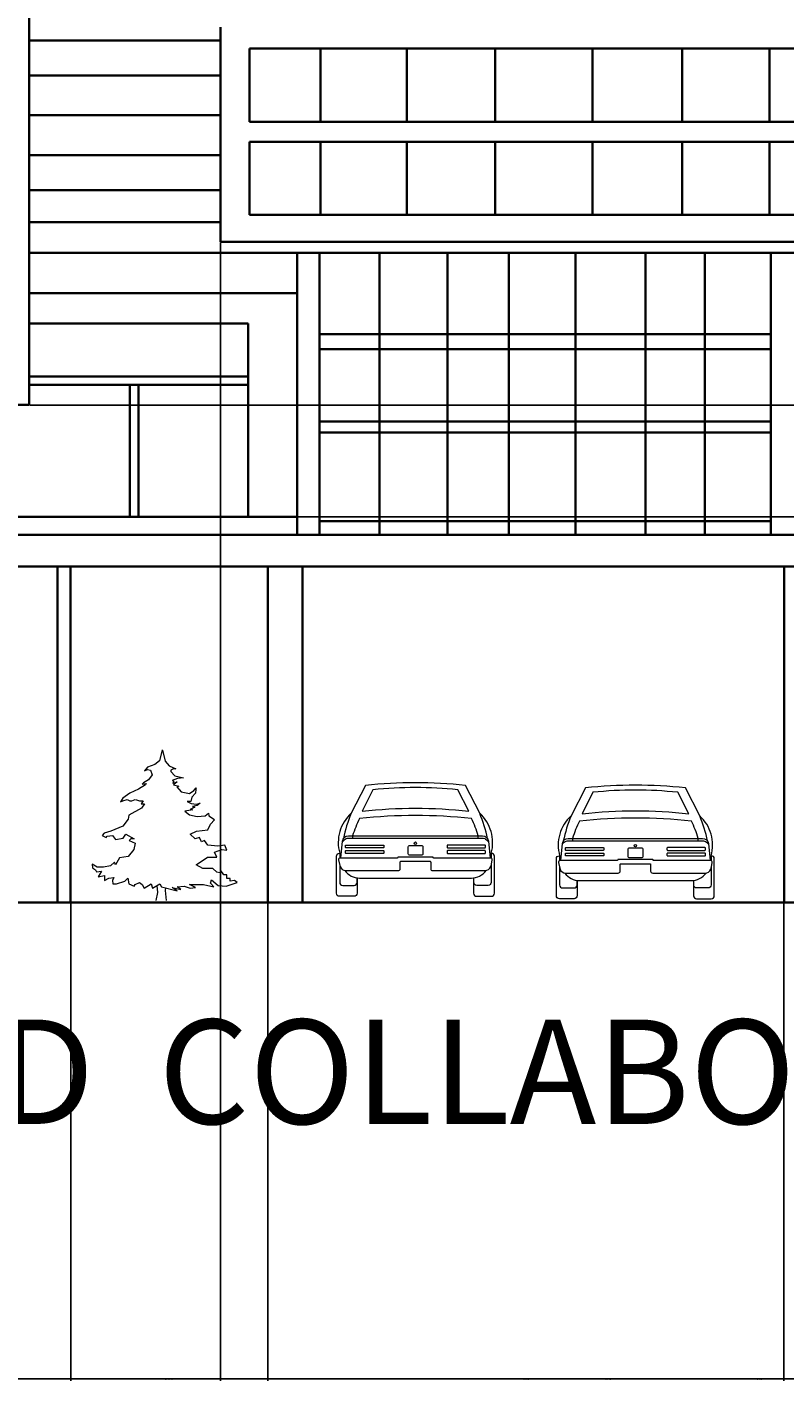
# Model space of a CAD drawing. Units: inches. Extents: x -160 to 434, y -145 to 103.
# Tile 4 of 7: x 107 to 176, y -145 to -22. Entities that reach past the tile are written whole.
import ezdxf

# ---------------------------------------------------------------- set-up
doc = ezdxf.new("R2010")
doc.units = ezdxf.units.IN
doc.header["$MEASUREMENT"] = 0
for name, color, linetype, lineweight in [('A-ANNO-DIMS', 2, 'Continuous', 18), ('A-ANNO-TEXT', 3, 'Continuous', 18), ('A-ELEV', 7, 'Continuous', 35), ('A-ENTO-VEHC', 8, 'Continuous', 13), ('L-PLNT', 3, 'Continuous', 13)]:
    doc.layers.add(name, color=color, linetype=linetype, lineweight=lineweight)
doc.styles.get("Standard").update_dxf_attribs({"font": 'arial.ttf'})
doc.dimstyles.get("Standard").update_dxf_attribs({"dimtxt": 0.18, "dimasz": 0.18, "dimexe": 0.18, "dimexo": 0.0625, "dimgap": 0.09, "dimtad": 0, "dimtih": 1, "dimtoh": 1, "dimdec": 4, "dimzin": 0, "dimdsep": 46, "dimtxsty": 'Standard', "dimcen": 0.09, "dimadec": 0, "dimazin": 0, "dimtfac": 1, "dimtdec": 4, "dimtofl": 0, "dimtmove": 0, "dimatfit": 3, "dimfxl": 1, "dimtolj": 1, "dimtzin": 0, "dimarcsym": 0})

# ---------------------------------------------------------------- blocks, each defined once
blk = doc.blocks.new('*U6')
for p, q in [((-24.66, 54.68), (-31.66, 40.93)), ((31.66, 40.93), (24.66, 54.68)), ((-30.95, 37.96), (-30.95, 37.96)), ((-37.32, 21.22), (-36.82, 18.83)), ((36.82, 18.83), (37.31, 21.2)), ((-27.55, 9), (27.55, 9))]:
    blk.add_line(p, q)
for points in [[(-20.92, 52.5), (-26.31, 41.89), (-26.31, 41.89, -0.059427), (26.31, 41.89), (20.92, 52.5, 0.05217)], [(-34.12, 25.29), (-15.92, 25.29, -0.414214), (-15.55, 24.92), (-15.55, 24.24, -0.414214), (-15.92, 23.87), (-34.12, 23.87, -0.414214), (-34.49, 24.24), (-34.49, 24.92, -0.414214)], [(-34.12, 22.54), (-15.92, 22.54, -0.414214), (-15.55, 22.17), (-15.55, 21.49, -0.414214), (-15.92, 21.12), (-34.12, 21.12, -0.414214), (-34.49, 21.49), (-34.49, 22.17, -0.414214)], [(-2.82, 25.12), (2.9, 25.12, -0.414214), (3.64, 24.38), (3.64, 20.97, -0.414214), (2.9, 20.23), (-2.82, 20.23, -0.414214), (-3.56, 20.97), (-3.56, 24.38, -0.414214)], [(34.12, 25.29), (15.92, 25.29, 0.414214), (15.55, 24.92), (15.55, 24.24, 0.414214), (15.92, 23.87), (34.12, 23.87, 0.414214), (34.49, 24.24), (34.49, 24.92, 0.414214)], [(34.12, 22.54), (15.92, 22.54, 0.414214), (15.55, 22.17), (15.55, 21.49, 0.414214), (15.92, 21.12), (34.12, 21.12, 0.414214), (34.49, 21.49), (34.49, 22.17, 0.414214)], [(-7.5, 16.83, -0.414214), (-7, 17.33), (7, 17.33, -0.414214), (7.5, 16.83), (7.5, 13.67, 0.414214), (8.5, 12.67), (34.29, 12.67, 0.322734), (37.1, 14.69, 0.029256), (37.41, 15.83), (37.84, 17.94, 0.475639), (37.12, 18.83), (9, 18.83, -0.414214), (8.75, 19.08, 0.414214), (8.5, 19.33), (-8.5, 19.33, 0.414214), (-8.75, 19.08, -0.414214), (-9, 18.83), (-37.12, 18.83, 0.475639), (-37.84, 17.94), (-37.41, 15.83, 0.029158), (-37.1, 14.7, 0.322842), (-34.29, 12.67), (-8.5, 12.67, 0.414214), (-7.5, 13.67)]]:
    blk.add_lwpolyline(points, format="xyb", close=True)
for points in [[(30.95, 28.64), (30.95, 29.82, 0.037308), (27.62, 38.34, 0.052989), (-27.62, 38.34, 0.037308), (-30.95, 29.82), (-30.95, 28.64)], [(-36.82, 18.83), (-35.99, 27.2, -0.380946), (-33.05, 29.82), (33.04, 29.82, -0.380474), (35.98, 27.2), (36.82, 18.83)], [(-36.02, 26.89), (-35.02, 27.89, -0.184023), (-33.05, 28.64), (33.05, 28.64, -0.184023), (35.02, 27.89), (36.02, 26.89)], [(-28.73, 9.08), (-28.73, 1.48, -0.414214), (-30.21, 0), (-37.44, 0, -0.414214), (-38.92, 1.48), (-38.92, 19.74, -0.414214), (-37.44, 21.22), (-37.32, 21.22)], [(28.67, 9.07), (28.67, 1.48, 0.414214), (30.15, 0), (37.38, 0, 0.414214), (38.86, 1.48), (38.86, 19.74, 0.414214), (37.38, 21.22), (37.32, 21.22)], [(-37.32, 15.44), (-37.32, 6.85, 0.414214), (-35.84, 5.37), (-30.21, 5.37, 0.414214), (-28.73, 6.85), (-28.73, 9.08)], [(37.32, 15.44), (37.32, 6.85, -0.414214), (35.84, 5.37), (30.21, 5.37, -0.414214), (28.73, 6.85), (28.73, 9.08)]]:
    blk.add_lwpolyline(points, format="xyb")
for points in [[(-37.32, 21.22), (-37.32, 18.8)], [(37.32, 21.22), (37.32, 18.8)]]:
    blk.add_lwpolyline(points)
blk.add_circle((0, 26.18), 0.596)
for centre, radius, start, end in [((0, -181.13), 237.1, 84.03003, 95.96997), ((-18.4, 26.45), 19.63, 132.48354, 195.46582), ((30.86, 14.66), 67.81, 157.21243, 168.23657), ((18.26, 26.38), 19.77, 344.85949, 47.35975), ((-31.75, 14.41), 68.72, 11.82698, 22.66251), ((-27.55, 17.88), 8.88, 215.57759, 270.00275), ((27.55, 17.88), 8.88, 270.00275, 324.39991)]:
    blk.add_arc(centre, radius, start, end)
blk = doc.blocks.new('*U7')
for p, q in [((-8.263, 7.598), (-8.747, 14.105)), ((-9.75, 0), (-8.263, 7.598)), ((-0.771, 9.56), (-0.69, 11.833)), ((0, 0), (-0.771, 9.56))]:
    blk.add_line(p, q)
for points in [[(-3.9, 142.35), (-6.596, 132.037), (-10.801, 128.443), (-17.81, 126.047), (-20.614, 122.452), (-17.81, 123.65), (-15.007, 123.051), (-13.605, 118.858), (-16.876, 114.065), (-21.549, 111.07), (-22.951, 109.872), (-19.212, 110.471), (-19.68, 109.273), (-26.222, 105.079), (-34.633, 101.485), (-41.175, 96.693), (-43.511, 93.098), (-41.175, 94.296), (-36.969, 95.494), (-34.633, 94.296), (-32.764, 94.296), (-29.493, 95.494)], [(-3.759, 141.97), (-1.074, 131.643), (2.437, 127.141), (8.84, 124.493), (6.568, 124.493), (4.09, 123.169), (4.296, 121.846), (7.807, 117.874), (16.069, 116.02), (10.492, 115.226), (5.535, 113.372), (6.981, 112.843), (5.948, 110.989), (10.286, 112.048), (6.775, 109.401), (11.732, 108.077), (9.873, 107.282), (13.797, 102.516), (21.852, 101.192), (25.983, 103.84), (28.048, 106.488), (27.842, 105.164), (27.429, 101.457), (24.124, 97.75), (23.091, 93.513), (19.58, 93.513), (23.505, 91.66), (28.255, 90.866), (31.973, 91.925), (29.081, 89.806), (24.537, 88.747), (26.809, 88.218), (22.472, 86.099), (24.95, 85.57), (17.308, 84.246), (21.852, 80.804), (29.081, 79.215), (36.723, 80.009), (39.821, 82.392), (40.028, 80.009), (45.398, 76.567)], [(-29.25, 95.55), (-25.287, 94.296), (-22.016, 94.296), (-23.885, 91.301), (-20.614, 91.301), (-23.418, 87.108), (-35.567, 80.518), (-36.035, 76.924), (-41.175, 70.334), (-52.389, 65.542), (-58.931, 63.744), (-60.8, 61.348), (-57.062, 59.551), (-56.128, 60.749), (-50.987, 61.348), (-48.184, 57.754), (-40.707, 58.952), (-38.371, 62.546), (-30.427, 58.353), (-33.698, 58.353), (-35.1, 56.556), (-29.493, 54.159), (-30.894, 48.169), (-36.035, 41.579), (-44.446, 40.381), (-48.184, 33.791), (-49.118, 36.188), (-52.857, 32.593), (-59.399, 31.395), (-65.473, 31.395), (-70.146, 34.39), (-69.679, 30.796), (-66.875, 28.999), (-65.941, 27.202), (-61.268, 27.801), (-64.539, 22.409), (-58.464, 23.607), (-58.464, 18.815), (-54.258, 21.211), (-49.586, 21.81), (-50.987, 18.815), (-50.52, 15.82), (-47.249, 15.82), (-39.306, 18.216), (-36.502, 21.211), (-35.567, 15.82), (-30.427, 13.423), (-29.493, 15.221), (-25.287, 17.018), (-22.951, 15.221), (-21.081, 11.626), (-14.539, 15.82), (-13.138, 11.626), (-6.128, 15.82), (-4.726, 12.824), (10.226, 9.23), (5.554, 12.225), (13.497, 10.428), (10.226, 12.824), (16.768, 13.423), (22.376, 11.626), (27.516, 12.225), (21.909, 15.221), (34.993, 15.221), (44.806, 12.824), (41.535, 16.419), (42.469, 19.414), (49.011, 14.023), (56.487, 13.423), (66.768, 17.018), (64.431, 18.815), (60.226, 18.216), (60.226, 20.612), (56.955, 20.612), (56.955, 24.206), (54.151, 24.206), (51.348, 28.4), (50.413, 26.004), (47.609, 26.603), (43.871, 30.197), (38.731, 30.197), (34.525, 30.197), (27.983, 33.791), (38.731, 40.98), (47.609, 40.98), (45.273, 45.773), (52.282, 48.169), (56.955, 47.57), (55.086, 52.362), (48.544, 51.164), (39.198, 52.362), (35.927, 56.556), (33.123, 55.357), (31.254, 59.551), (27.049, 58.353), (22.376, 62.546), (28.451, 65.542), (39.198, 66.74), (41.535, 72.131), (45.273, 76.325)]]:
    blk.add_lwpolyline(points)
blk = doc.blocks.new('*D12')
at = {"layer": 'A-ANNO-DIMS', "color": 0, "lineweight": -2, "transparency": 16777216}
for p, q in [((-84.07, -101.41), (-84.07, -144.81)), ((403.75, -101.41), (403.75, -144.81)), ((-83.89, -144.63), (159.44, -144.63)), ((403.57, -144.63), (160.24, -144.63))]:
    blk.add_line(p, q, dxfattribs=at)
at = {"layer": 'A-ANNO-DIMS', "color": 0, "transparency": 16777216}
for points in [[(-83.89, -144.6), (-83.89, -144.66), (-84.07, -144.63)], [(403.57, -144.6), (403.57, -144.66), (403.75, -144.63)]]:
    blk.add_solid(points, dxfattribs=at)
at = {"layer": 'Defpoints', "color": 0, "transparency": 16777216}
for p in [(-84.07, -101.35), (403.75, -101.35), (403.75, -144.63)]:
    blk.add_point(p, dxfattribs=at)
at = {"layer": 'A-ANNO-DIMS', "color": 0, "transparency": 16777216, "insert": (159.84, -144.63), "char_height": 0.18, "attachment_point": 5}
blk.add_mtext('\\A1;487.8', dxfattribs=at)
blk = doc.blocks.new('*D19')
at = {"layer": 'A-ANNO-DIMS', "color": 0, "lineweight": -2, "transparency": 16777216}
for p, q in [((74.92, -101.41), (74.92, -144.81)), ((111.05, -101.41), (111.05, -144.81)), ((75.1, -144.63), (92.59, -144.63)), ((110.87, -144.63), (93.38, -144.63))]:
    blk.add_line(p, q, dxfattribs=at)
at = {"layer": 'A-ANNO-DIMS', "color": 0, "transparency": 16777216}
for points in [[(75.1, -144.6), (75.1, -144.66), (74.92, -144.63)], [(110.87, -144.6), (110.87, -144.66), (111.05, -144.63)]]:
    blk.add_solid(points, dxfattribs=at)
at = {"layer": 'Defpoints', "color": 0, "transparency": 16777216}
for p in [(74.92, -101.35), (111.05, -101.35), (111.05, -144.63)]:
    blk.add_point(p, dxfattribs=at)
at = {"layer": 'A-ANNO-DIMS', "color": 0, "transparency": 16777216, "insert": (92.98, -144.63), "char_height": 0.18, "attachment_point": 5}
blk.add_mtext('\\A1;36.12', dxfattribs=at)
blk = doc.blocks.new('*D20')
at = {"layer": 'A-ANNO-DIMS', "color": 0, "lineweight": -2, "transparency": 16777216}
for p, q in [((111.05, -101.41), (111.05, -144.81)), ((128.95, -101.41), (128.95, -144.81)), ((111.23, -144.63), (119.54, -144.63)), ((128.77, -144.63), (120.45, -144.63))]:
    blk.add_line(p, q, dxfattribs=at)
at = {"layer": 'A-ANNO-DIMS', "color": 0, "transparency": 16777216}
for points in [[(111.23, -144.6), (111.23, -144.66), (111.05, -144.63)], [(128.77, -144.6), (128.77, -144.66), (128.95, -144.63)]]:
    blk.add_solid(points, dxfattribs=at)
at = {"layer": 'Defpoints', "color": 0, "transparency": 16777216}
for p in [(111.05, -101.35), (128.95, -101.35), (128.95, -144.63)]:
    blk.add_point(p, dxfattribs=at)
at = {"layer": 'A-ANNO-DIMS', "color": 0, "transparency": 16777216, "insert": (120, -144.63), "char_height": 0.18, "attachment_point": 5}
blk.add_mtext('\\A1;17.907', dxfattribs=at)
blk = doc.blocks.new('*D21')
at = {"layer": 'A-ANNO-DIMS', "color": 0, "lineweight": -2, "transparency": 16777216}
for p, q in [((128.95, -101.41), (128.95, -144.81)), ((175.81, -101.41), (175.81, -144.81)), ((129.13, -144.63), (151.99, -144.63)), ((175.63, -144.63), (152.78, -144.63))]:
    blk.add_line(p, q, dxfattribs=at)
at = {"layer": 'A-ANNO-DIMS', "color": 0, "transparency": 16777216}
for points in [[(129.13, -144.6), (129.13, -144.66), (128.95, -144.63)], [(175.63, -144.6), (175.63, -144.66), (175.81, -144.63)]]:
    blk.add_solid(points, dxfattribs=at)
at = {"layer": 'Defpoints', "color": 0, "transparency": 16777216}
for p in [(128.95, -101.35), (175.81, -101.35), (175.81, -144.63)]:
    blk.add_point(p, dxfattribs=at)
at = {"layer": 'A-ANNO-DIMS', "color": 0, "transparency": 16777216, "insert": (152.38, -144.63), "char_height": 0.18, "attachment_point": 5}
blk.add_mtext('\\A1;46.86', dxfattribs=at)
blk = doc.blocks.new('*D22')
at = {"layer": 'A-ANNO-DIMS', "color": 0, "lineweight": -2, "transparency": 16777216}
for p, q in [((175.81, -101.41), (175.81, -144.81)), ((216.81, -101.09), (216.81, -144.81)), ((175.99, -144.63), (195.91, -144.63)), ((216.63, -144.63), (196.71, -144.63))]:
    blk.add_line(p, q, dxfattribs=at)
at = {"layer": 'A-ANNO-DIMS', "color": 0, "transparency": 16777216}
for points in [[(175.99, -144.6), (175.99, -144.66), (175.81, -144.63)], [(216.63, -144.6), (216.63, -144.66), (216.81, -144.63)]]:
    blk.add_solid(points, dxfattribs=at)
at = {"layer": 'Defpoints', "color": 0, "transparency": 16777216}
for p in [(175.81, -101.35), (216.81, -101.02), (216.81, -144.63)]:
    blk.add_point(p, dxfattribs=at)
at = {"layer": 'A-ANNO-DIMS', "color": 0, "transparency": 16777216, "insert": (196.31, -144.63), "char_height": 0.18, "attachment_point": 5}
blk.add_mtext('\\A1;40.99', dxfattribs=at)
blk = doc.blocks.new('*D31')
at = {"layer": 'A-ANNO-DIMS', "color": 0, "lineweight": -2, "transparency": 16777216}
for p, q in [((107.33, 8.95), (433.98, 8.95)), ((433.8, 8.77), (433.8, -23.43)), ((433.8, -55.99), (433.8, -23.79)), ((107.33, -56.17), (433.98, -56.17))]:
    blk.add_line(p, q, dxfattribs=at)
at = {"layer": 'A-ANNO-DIMS', "color": 0, "transparency": 16777216}
for points in [[(433.77, 8.77), (433.83, 8.77), (433.8, 8.95)], [(433.77, -55.99), (433.83, -55.99), (433.8, -56.17)]]:
    blk.add_solid(points, dxfattribs=at)
at = {"layer": 'Defpoints', "color": 0, "transparency": 16777216}
for p in [(107.27, 8.95), (107.27, -56.17), (433.8, -56.17)]:
    blk.add_point(p, dxfattribs=at)
at = {"layer": 'A-ANNO-DIMS', "color": 0, "transparency": 16777216, "insert": (433.8, -23.61), "char_height": 0.18, "attachment_point": 5}
blk.add_mtext('\\A1;65.11', dxfattribs=at)
blk = doc.blocks.new('*D32')
at = {"layer": 'A-ANNO-DIMS', "color": 0, "lineweight": -2, "transparency": 16777216}
for p, q in [((107.33, -56.17), (433.98, -56.17)), ((433.8, -56.35), (433.8, -61.07)), ((433.8, -66.15), (433.8, -61.43)), ((106.73, -66.33), (433.98, -66.33))]:
    blk.add_line(p, q, dxfattribs=at)
at = {"layer": 'A-ANNO-DIMS', "color": 0, "transparency": 16777216}
for points in [[(433.77, -56.35), (433.83, -56.35), (433.8, -56.17)], [(433.77, -66.15), (433.83, -66.15), (433.8, -66.33)]]:
    blk.add_solid(points, dxfattribs=at)
at = {"layer": 'Defpoints', "color": 0, "transparency": 16777216}
for p in [(107.27, -56.17), (106.67, -66.33), (433.8, -66.33)]:
    blk.add_point(p, dxfattribs=at)
at = {"layer": 'A-ANNO-DIMS', "color": 0, "transparency": 16777216, "insert": (433.8, -61.25), "char_height": 0.18, "attachment_point": 5}
blk.add_mtext('\\A1;10.165', dxfattribs=at)
blk = doc.blocks.new('*D41')
at = {"layer": 'A-ANNO-DIMS', "color": 0, "lineweight": -2, "transparency": 16777216}
for p, q in [((124.65, -41.4), (124.65, -144.81)), ((222.55, -41.85), (222.55, -144.81)), ((124.83, -144.63), (173.28, -144.63)), ((222.37, -144.63), (173.93, -144.63))]:
    blk.add_line(p, q, dxfattribs=at)
at = {"layer": 'A-ANNO-DIMS', "color": 0, "transparency": 16777216}
for points in [[(124.83, -144.6), (124.83, -144.66), (124.65, -144.63)], [(222.37, -144.6), (222.37, -144.66), (222.55, -144.63)]]:
    blk.add_solid(points, dxfattribs=at)
at = {"layer": 'Defpoints', "color": 0, "transparency": 16777216}
for p in [(124.65, -41.34), (222.55, -41.79), (222.55, -144.63)]:
    blk.add_point(p, dxfattribs=at)
at = {"layer": 'A-ANNO-DIMS', "color": 0, "transparency": 16777216, "insert": (173.6, -144.63), "char_height": 0.18, "attachment_point": 5}
blk.add_mtext('\\A1;97.9', dxfattribs=at)

msp = doc.modelspace()

# ---------------------------------------------------------------- linework, layer by layer
at = {"layer": 'A-ELEV'}
for p, q in [((107.2684, 8.9457), (107.2684, -38.311)), ((124.6537, -21.8399), (124.6537, -41.3403)), ((107.2684, -23.0465), (124.6537, -23.0465)), ((127.2839, -25.5804), (127.2839, -23.7966)), ((127.2839, -23.7966), (128.7392, -23.7966)), ((137.8943, -23.7966), (128.7392, -23.7966)), ((133.7225, -23.7966), (133.7225, -30.4469)), ((219.5071, -23.7966), (137.8943, -23.7966)), ((141.5547, -23.7966), (141.5547, -30.4469)), ((149.5831, -23.7966), (149.5831, -30.4469)), ((158.4144, -23.7966), (158.4144, -30.4469)), ((166.5644, -23.7966), (166.5644, -30.4469)), ((174.4858, -23.7966), (174.4858, -30.4469)), ((127.2839, -25.5804), (127.2839, -30.4469)), ((107.2684, -26.2352), (124.6537, -26.2352)), ((107.2684, -29.849), (124.6537, -29.849)), ((127.2839, -30.4469), (128.7392, -30.4469)), ((137.8943, -30.4469), (128.7392, -30.4469)), ((219.5071, -30.4469), (137.8943, -30.4469)), ((127.2839, -32.2746), (128.7392, -32.2746)), ((127.2839, -32.2746), (127.2839, -37.8491)), ((137.8943, -32.2746), (128.7392, -32.2746)), ((133.7225, -32.2746), (133.7225, -38.9063)), ((219.5071, -32.2746), (137.8943, -32.2746)), ((141.5547, -32.2746), (141.5547, -38.9063)), ((149.5831, -32.2746), (149.5831, -38.9063)), ((158.4144, -32.2746), (158.4144, -38.9063)), ((166.5644, -32.2746), (166.5644, -38.9063)), ((174.4858, -32.2746), (174.4858, -38.9063)), ((107.2684, -33.4628), (124.6537, -33.4628)), ((107.2684, -36.6515), (124.6537, -36.6515)), ((127.2839, -38.9063), (127.2839, -37.8491)), ((107.2684, -56.1669), (107.2684, -38.311)), ((128.7392, -38.9063), (127.2839, -38.9063)), ((128.7392, -38.9063), (137.8943, -38.9063)), ((219.5071, -38.9063), (137.8943, -38.9063)), ((107.2684, -39.5641), (124.6537, -39.5641)), ((124.6537, -41.3403), (137.8943, -41.3403)), ((213.3013, -41.3403), (137.8943, -41.3403)), ((107.2684, -42.3312), (134.424, -42.3312)), ((131.6105, -46.0109), (131.6105, -42.3312)), ((133.6491, -42.3312), (133.6491, -67.9742)), ((134.424, -42.3312), (222.5284, -42.3312)), ((139.101, -42.3312), (139.101, -67.9742)), ((145.2682, -42.3312), (145.2682, -67.9742)), ((150.8243, -42.3312), (150.8243, -67.9742)), ((156.8803, -42.3312), (156.8803, -67.9742)), ((163.228, -42.3312), (163.228, -67.9742)), ((168.6173, -42.3312), (168.6173, -67.9742)), ((174.6035, -42.3312), (174.6035, -67.9742)), ((107.2684, -46.0109), (131.6105, -46.0109)), ((131.6105, -46.0109), (131.6105, -67.9742)), ((107.2684, -48.7744), (127.1729, -48.7744)), ((127.1729, -48.7744), (127.1729, -66.3322)), ((174.6035, -49.7355), (133.6491, -49.7355)), ((174.6035, -51.1087), (133.6491, -51.1087)), ((107.2684, -53.5674), (127.1729, -53.5674)), ((107.2684, -54.3391), (127.1729, -54.3391)), ((116.4049, -54.3391), (116.4049, -66.3322)), ((117.1995, -54.3391), (117.1995, -66.3322)), ((78.691, -56.1669), (107.2684, -56.1669)), ((174.6035, -57.6699), (133.6491, -57.6699)), ((174.6035, -58.6768), (133.6491, -58.6768)), ((55.5639, -66.3322), (131.6105, -66.3322)), ((174.6035, -66.7321), (133.6491, -66.7321)), ((2.6577, -67.9742), (206.9244, -67.9742)), ((2.6577, -70.8373), (206.9244, -70.8373)), ((109.8513, -70.8373), (109.8513, -101.346)), ((111.0454, -70.8373), (111.0454, -101.346)), ((128.9529, -70.8373), (128.9529, -101.346)), ((132.1013, -70.8373), (132.1013, -101.346)), ((175.8147, -70.8373), (175.8147, -101.346)), ((2.6577, -101.346), (403.7477, -101.346))]:
    msp.add_line(p, q, dxfattribs=at)

# ---------------------------------------------------------------- block references
at = {"layer": 'A-ENTO-VEHC', "xscale": 0.1843091790693797, "yscale": 0.1843091790693797, "zscale": 0.1843091790693797}
for p in [(142.3516, -100.7948), (162.3232, -101.0241)]:
    msp.add_blockref('*U6', p, dxfattribs=at)
at = {"layer": 'L-PLNT', "xscale": 0.0961203238098615, "yscale": 0.0961203238098615, "zscale": 0.0961203238098615}
msp.add_blockref('*U7', (119.7413, -101.1712), dxfattribs=at)

# ---------------------------------------------------------------- texts
at = {"layer": 'A-ANNO-TEXT'}
msp.add_text('FRONT   ELEVATION - RESEARCH   SPINE   AND  COLLABORATION   PODS  (NEW   CONCEPT)', height=9.480943, dxfattribs=at).set_placement((-160.9184, -121.4719))

# ---------------------------------------------------------------- dimensions: what is measured, and where the dimension line sits
at = {"layer": 'A-ANNO-DIMS'}
for base, p1, p2, override, picture, middle in [((433.7977, -56.1669), (107.2684, 8.9457), (107.2684, -56.1669), {"dimdec": 2, "dimlfac": 1, "dimrnd": 0, "dimzin": 0, "dimdsep": 46, "dimlunit": 2}, '*D31', (433.7977, -23.6106)), ((433.7977, -66.3322), (107.2684, -56.1669), (106.6672, -66.3322), {"dimdec": 3, "dimlfac": 1, "dimrnd": 0, "dimzin": 0, "dimdsep": 46, "dimlunit": 2}, '*D32', (433.7977, -61.2496))]:
    dim = msp.add_linear_dim(base=base, p1=p1, p2=p2, angle=90, dimstyle='Standard', override=override, dxfattribs=at)
    dim.commit()
    dim.dimension.update_dxf_attribs({"geometry": picture, "text_midpoint": middle})
for base, p1, p2, override, picture, middle in [((222.553, -144.6322), (124.6537, -41.3403), (222.553, -41.7856), {"dimdec": 1, "dimlfac": 1, "dimrnd": 0, "dimzin": 0, "dimdsep": 46, "dimlunit": 2}, '*D41', (173.6034, -144.6322)), ((403.7477, -144.6322), (-84.0722, -101.346), (403.7477, -101.346), {"dimdec": 1, "dimlfac": 1, "dimrnd": 0, "dimzin": 0, "dimdsep": 46, "dimlunit": 2}, '*D12', (159.8378, -144.6322)), ((111.0454, -144.6322), (74.9222, -101.346), (111.0454, -101.346), {"dimdec": 2, "dimlfac": 1, "dimrnd": 0, "dimzin": 0, "dimdsep": 46, "dimlunit": 2}, '*D19', (92.9838, -144.6322)), ((128.9529, -144.63222), (111.04541, -101.34605), (128.9529, -101.34605), {"dimdec": 3, "dimlfac": 1, "dimrnd": 0, "dimzin": 0, "dimdsep": 46, "dimlunit": 2}, '*D20', (119.99916, -144.63222)), ((175.8147, -144.6322), (128.9529, -101.346), (175.8147, -101.346), {"dimdec": 2, "dimlfac": 1, "dimrnd": 0, "dimzin": 0, "dimdsep": 46, "dimlunit": 2}, '*D21', (152.3838, -144.6322)), ((216.8055, -144.6322), (175.8147, -101.346), (216.8055, -101.0241), {"dimdec": 2, "dimlfac": 1, "dimrnd": 0, "dimzin": 0, "dimdsep": 46, "dimlunit": 2}, '*D22', (196.3101, -144.6322))]:
    dim = msp.add_linear_dim(base=base, p1=p1, p2=p2, dimstyle='Standard', override=override, dxfattribs=at)
    dim.commit()
    dim.dimension.update_dxf_attribs({"geometry": picture, "text_midpoint": middle})

doc.saveas('drawing.dxf')
